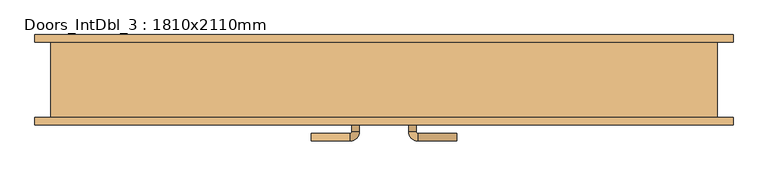
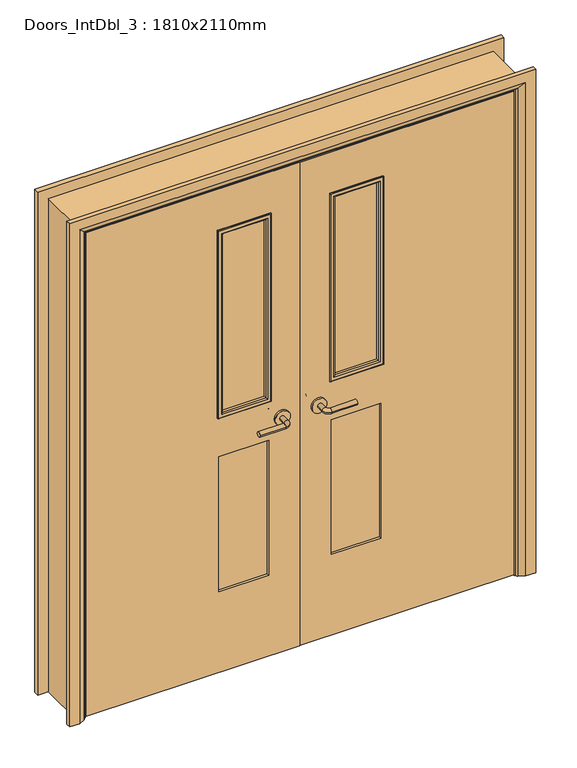
"""IFC4 building model written with IfcOpenShell, lengths in millimetres: door geometry, Doors_IntDbl_3 : 1810x2110mm."""

from ifc_helpers import new_model, si_unit, point, frame, frame_2d, origin, place, context, project, spatial, polyline, circle_curve, ellipse_curve, trimmed, segment, composite_curve, outline, extrude, faceted_brep, source, transform, mapped, element, save
from ifc_brep_helpers import plane_surface, cylinder_surface, revolved_surface, advanced_brep


def doors_intdbl_3_1810x2110mm_301b02ef(model_context):
    return source(origin(), model_context, "Body", "SolidModel", [
        advanced_brep(
        [(-66.5, -61.6, 1007.0), (-86.5, -61.6, 1007.0), (-86.5, -31.6, 1007.0), (-66.5, -31.6, 1007.0), (-91.5, -26.6, 1007.0), (-91.5, -6.6, 1007.0), (-196.5, -6.6, 1007.0), (-196.5, -26.6, 1007.0)],
        [
            (0, 1, circle_curve(frame((-76.5, -61.6, 1007.0), z_axis=(0.0, -1.0, 0.0), x_axis=(-1.0, 0.0, 0.0)), 10.0)),
            (1, 0, circle_curve(frame((-76.5, -61.6, 1007.0), z_axis=(0.0, -1.0, 0.0), x_axis=(-1.0, 0.0, 0.0)), 10.0)),
            (1, 2),
            (2, 3, circle_curve(frame((-76.5, -31.6, 1007.0), z_axis=(0.0, -1.0, 0.0), x_axis=(-1.0, 0.0, 0.0)), 10.0)),
            (3, 0),
            (3, 2, circle_curve(frame((-76.5, -31.6, 1007.0), z_axis=(0.0, -1.0, 0.0), x_axis=(-1.0, 0.0, 0.0)), 10.0)),
            (4, 5, circle_curve(frame((-91.5, -16.6, 1007.0), z_axis=(1.0, 0.0, 0.0), x_axis=(0.0, -1.0, 0.0)), 10.0)),
            (5, 3, circle_curve(frame((-91.5, -31.6, 1007.0), z_axis=(0.0, 0.0, -1.0), x_axis=(1.0, 0.0, 0.0)), 25.0)),
            (2, 4, circle_curve(frame((-91.5, -31.6, 1007.0), z_axis=(0.0, 0.0, 1.0), x_axis=(1.0, 0.0, 0.0)), 5.0)),
            (5, 4, circle_curve(frame((-91.5, -16.6, 1007.0), z_axis=(1.0, 0.0, 0.0), x_axis=(0.0, -1.0, 0.0)), 10.0)),
            (6, 7, circle_curve(frame((-196.5, -16.6, 1007.0), z_axis=(-1.0, 0.0, 0.0), x_axis=(0.0, -1.0, 0.0)), 10.0)),
            (7, 6, circle_curve(frame((-196.5, -16.6, 1007.0), z_axis=(-1.0, 0.0, 0.0), x_axis=(0.0, -1.0, 0.0)), 10.0)),
            (4, 7),
            (6, 5),
        ],
        [
            plane_surface(frame((-76.5, -61.6, 1007.0), z_axis=(0.0, -1.0, 0.0), x_axis=(0.0, 0.0, 1.0))),
            cylinder_surface(frame((-76.5, -61.6, 1007.0), z_axis=(0.0, -1.0, 0.0), x_axis=(-1.0, 0.0, 0.0)), 10.0),
            revolved_surface(trimmed(ellipse_curve(frame((-76.5, -31.6, 1007.0), z_axis=(0.0, 1.0, 0.0), x_axis=(-1.0, 0.0, 0.0)), 10.0, 10.0), [point((-66.5, -31.6, 1007.0))], [point((-86.5, -31.6, 1007.0))], True, "CARTESIAN"), (-91.5, -31.6, 1007.0), (0.0, 0.0, -1.0)),
            revolved_surface(trimmed(ellipse_curve(frame((-76.5, -31.6, 1007.0), z_axis=(0.0, 1.0, 0.0), x_axis=(-1.0, 0.0, 0.0)), 10.0, 10.0), [point((-86.5, -31.6, 1007.0))], [point((-66.5, -31.6, 1007.0))], True, "CARTESIAN"), (-91.5, -31.6, 1007.0), (0.0, 0.0, -1.0)),
            plane_surface(frame((-196.5, -16.6, 1007.0), z_axis=(-1.0, 0.0, 0.0), x_axis=(0.0, 0.0, 1.0))),
            cylinder_surface(frame((-91.5, -16.6, 1007.0), z_axis=(1.0, 0.0, 0.0), x_axis=(0.0, -1.0, 0.0)), 10.0),
        ],
        [
            (0, [[1, 2]]),
            (1, [[3, 4, 5, -2]]),
            (1, [[-5, 6, -3, -1]]),
            (2, [[7, 8, -4, 9]]),
            (3, [[10, -9, -6, -8]]),
            (4, [[11, 12]]),
            (5, [[13, -11, 14, -7]]),
            (5, [[-14, -12, -13, -10]]),
        ],
    ),
        extrude(outline(composite_curve([segment(trimmed(circle_curve(frame_2d((1007.0, -74.0)), 30.0), [point((1007.0, -44.0))], [point((1007.0, -104.0))], False, "CARTESIAN"), True, "CONTINUOUS"), segment(trimmed(circle_curve(frame_2d((1007.0, -74.0)), 30.0), [point((1007.0, -104.0))], [point((1007.0, -44.0))], False, "CARTESIAN"), True, "CONTINUOUS")], self_intersect=False)), frame((0.0, -69.6, 0.0), z_axis=(0.0, 1.0, 0.0), x_axis=(0.0, 0.0, 1.0)), (0.0, 0.0, 1.0), 8.0),
        advanced_brep(
        [(-66.5, -109.6, 1007.0), (-86.5, -109.6, 1007.0), (-66.5, -139.6, 1007.0), (-86.5, -139.6, 1007.0), (-91.5, -144.6, 1007.0), (-91.5, -164.6, 1007.0), (-196.5, -164.6, 1007.0), (-196.5, -144.6, 1007.0)],
        [
            (0, 1, circle_curve(frame((-76.5, -109.6, 1007.0), z_axis=(0.0, 1.0, 0.0), x_axis=(-1.0, 0.0, 0.0)), 10.0)),
            (1, 0, circle_curve(frame((-76.5, -109.6, 1007.0), z_axis=(0.0, 1.0, 0.0), x_axis=(-1.0, 0.0, 0.0)), 10.0)),
            (0, 2),
            (2, 3, circle_curve(frame((-76.5, -139.6, 1007.0), z_axis=(0.0, 1.0, 0.0), x_axis=(-1.0, 0.0, 0.0)), 10.0)),
            (3, 1),
            (3, 2, circle_curve(frame((-76.5, -139.6, 1007.0), z_axis=(0.0, 1.0, 0.0), x_axis=(-1.0, 0.0, 0.0)), 10.0)),
            (4, 3, circle_curve(frame((-91.5, -139.6, 1007.0), z_axis=(0.0, 0.0, 1.0), x_axis=(1.0, 0.0, 0.0)), 5.0)),
            (2, 5, circle_curve(frame((-91.5, -139.6, 1007.0), z_axis=(0.0, 0.0, -1.0), x_axis=(1.0, 0.0, 0.0)), 25.0)),
            (5, 4, circle_curve(frame((-91.5, -154.6, 1007.0), z_axis=(1.0, 0.0, 0.0), x_axis=(0.0, 1.0, 0.0)), 10.0)),
            (4, 5, circle_curve(frame((-91.5, -154.6, 1007.0), z_axis=(1.0, 0.0, 0.0), x_axis=(0.0, 1.0, 0.0)), 10.0)),
            (6, 7, circle_curve(frame((-196.5, -154.6, 1007.0), z_axis=(-1.0, 0.0, 0.0), x_axis=(0.0, 1.0, 0.0)), 10.0)),
            (7, 6, circle_curve(frame((-196.5, -154.6, 1007.0), z_axis=(-1.0, 0.0, 0.0), x_axis=(0.0, 1.0, 0.0)), 10.0)),
            (5, 6),
            (7, 4),
        ],
        [
            plane_surface(frame((-76.5, -109.6, 1007.0), z_axis=(0.0, 1.0, 0.0), x_axis=(0.0, 0.0, 1.0))),
            cylinder_surface(frame((-76.5, -109.6, 1007.0), z_axis=(0.0, 1.0, 0.0), x_axis=(-1.0, 0.0, 0.0)), 10.0),
            revolved_surface(trimmed(ellipse_curve(frame((-76.5, -139.6, 1007.0), z_axis=(0.0, 1.0, 0.0), x_axis=(-1.0, 0.0, 0.0)), 10.0, 10.0), [point((-66.5, -139.6, 1007.0))], [point((-86.5, -139.6, 1007.0))], True, "CARTESIAN"), (-91.5, -139.6, 1007.0), (0.0, 0.0, -1.0)),
            revolved_surface(trimmed(ellipse_curve(frame((-76.5, -139.6, 1007.0), z_axis=(0.0, 1.0, 0.0), x_axis=(-1.0, 0.0, 0.0)), 10.0, 10.0), [point((-86.5, -139.6, 1007.0))], [point((-66.5, -139.6, 1007.0))], True, "CARTESIAN"), (-91.5, -139.6, 1007.0), (0.0, 0.0, -1.0)),
            plane_surface(frame((-196.5, -154.6, 1007.0), z_axis=(-1.0, 0.0, 0.0), x_axis=(0.0, 0.0, 1.0))),
            cylinder_surface(frame((-91.5, -154.6, 1007.0), z_axis=(1.0, 0.0, 0.0), x_axis=(0.0, 1.0, 0.0)), 10.0),
        ],
        [
            (0, [[1, 2]]),
            (1, [[-1, 3, 4, 5]]),
            (1, [[-2, -5, 6, -3]]),
            (2, [[7, -4, 8, 9]]),
            (3, [[-8, -6, -7, 10]]),
            (4, [[11, 12]]),
            (5, [[-9, 13, -12, 14]]),
            (5, [[-10, -14, -11, -13]]),
        ],
    ),
        extrude(outline(composite_curve([segment(trimmed(circle_curve(frame_2d((1007.0, -74.0)), 30.0), [point((1007.0, -44.0))], [point((1007.0, -104.0))], False, "CARTESIAN"), True, "CONTINUOUS"), segment(trimmed(circle_curve(frame_2d((1007.0, -74.0)), 30.0), [point((1007.0, -104.0))], [point((1007.0, -44.0))], False, "CARTESIAN"), True, "CONTINUOUS")], self_intersect=False)), frame((0.0, -109.6, 0.0), z_axis=(0.0, 1.0, 0.0), x_axis=(0.0, 0.0, 1.0)), (0.0, 0.0, 1.0), 8.0),
        advanced_brep(
        [(66.5, -61.6, 1007.0), (86.5, -61.6, 1007.0), (66.5, -31.6, 1007.0), (86.5, -31.6, 1007.0), (91.5, -26.6, 1007.0), (91.5, -6.6, 1007.0), (196.5, -6.6, 1007.0), (196.5, -26.6, 1007.0)],
        [
            (0, 1, circle_curve(frame((76.5, -61.6, 1007.0), z_axis=(0.0, -1.0, 0.0), x_axis=(1.0, 0.0, 0.0)), 10.0)),
            (1, 0, circle_curve(frame((76.5, -61.6, 1007.0), z_axis=(0.0, -1.0, 0.0), x_axis=(1.0, 0.0, 0.0)), 10.0)),
            (0, 2),
            (2, 3, circle_curve(frame((76.5, -31.6, 1007.0), z_axis=(0.0, -1.0, 0.0), x_axis=(1.0, 0.0, 0.0)), 10.0)),
            (3, 1),
            (3, 2, circle_curve(frame((76.5, -31.6, 1007.0), z_axis=(0.0, -1.0, 0.0), x_axis=(1.0, 0.0, 0.0)), 10.0)),
            (4, 3, circle_curve(frame((91.5, -31.6, 1007.0), z_axis=(0.0, 0.0, 1.0), x_axis=(-1.0, 0.0, 0.0)), 5.0)),
            (2, 5, circle_curve(frame((91.5, -31.6, 1007.0), z_axis=(0.0, 0.0, -1.0), x_axis=(-1.0, 0.0, 0.0)), 25.0)),
            (5, 4, circle_curve(frame((91.5, -16.6, 1007.0), z_axis=(-1.0, 0.0, 0.0), x_axis=(0.0, -1.0, 0.0)), 10.0)),
            (4, 5, circle_curve(frame((91.5, -16.6, 1007.0), z_axis=(-1.0, 0.0, 0.0), x_axis=(0.0, -1.0, 0.0)), 10.0)),
            (6, 7, circle_curve(frame((196.5, -16.6, 1007.0), z_axis=(1.0, 0.0, 0.0), x_axis=(0.0, -1.0, 0.0)), 10.0)),
            (7, 6, circle_curve(frame((196.5, -16.6, 1007.0), z_axis=(1.0, 0.0, 0.0), x_axis=(0.0, -1.0, 0.0)), 10.0)),
            (5, 6),
            (7, 4),
        ],
        [
            plane_surface(frame((76.5, -61.6, 1007.0), z_axis=(0.0, -1.0, 0.0), x_axis=(0.0, 0.0, 1.0))),
            cylinder_surface(frame((76.5, -61.6, 1007.0), z_axis=(0.0, -1.0, 0.0), x_axis=(1.0, 0.0, 0.0)), 10.0),
            revolved_surface(trimmed(ellipse_curve(frame((76.5, -31.6, 1007.0), z_axis=(0.0, -1.0, 0.0), x_axis=(1.0, 0.0, 0.0)), 10.0, 10.0), [point((66.5, -31.6, 1007.0))], [point((86.5, -31.6, 1007.0))], True, "CARTESIAN"), (91.5, -31.6, 1007.0), (0.0, 0.0, -1.0)),
            revolved_surface(trimmed(ellipse_curve(frame((76.5, -31.6, 1007.0), z_axis=(0.0, -1.0, 0.0), x_axis=(1.0, 0.0, 0.0)), 10.0, 10.0), [point((86.5, -31.6, 1007.0))], [point((66.5, -31.6, 1007.0))], True, "CARTESIAN"), (91.5, -31.6, 1007.0), (0.0, 0.0, -1.0)),
            plane_surface(frame((196.5, -16.6, 1007.0), z_axis=(1.0, 0.0, 0.0), x_axis=(0.0, 0.0, 1.0))),
            cylinder_surface(frame((91.5, -16.6, 1007.0), z_axis=(-1.0, 0.0, 0.0), x_axis=(0.0, -1.0, 0.0)), 10.0),
        ],
        [
            (0, [[1, 2]]),
            (1, [[-1, 3, 4, 5]]),
            (1, [[-2, -5, 6, -3]]),
            (2, [[7, -4, 8, 9]]),
            (3, [[-8, -6, -7, 10]]),
            (4, [[11, 12]]),
            (5, [[-9, 13, -12, 14]]),
            (5, [[-10, -14, -11, -13]]),
        ],
    ),
        extrude(outline(composite_curve([segment(trimmed(circle_curve(frame_2d((1007.0, 74.0)), 30.0), [point((1007.0, 44.0))], [point((1007.0, 104.0))], False, "CARTESIAN"), True, "CONTINUOUS"), segment(trimmed(circle_curve(frame_2d((1007.0, 74.0)), 30.0), [point((1007.0, 104.0))], [point((1007.0, 44.0))], False, "CARTESIAN"), True, "CONTINUOUS")], self_intersect=False)), frame((0.0, -69.6, 0.0), z_axis=(0.0, 1.0, 0.0), x_axis=(0.0, 0.0, 1.0)), (0.0, 0.0, 1.0), 8.0),
        advanced_brep(
        [(66.5, -109.6, 1007.0), (86.5, -109.6, 1007.0), (86.5, -139.6, 1007.0), (66.5, -139.6, 1007.0), (91.5, -144.6, 1007.0), (91.5, -164.6, 1007.0), (196.5, -164.6, 1007.0), (196.5, -144.6, 1007.0)],
        [
            (0, 1, circle_curve(frame((76.5, -109.6, 1007.0), z_axis=(0.0, 1.0, 0.0), x_axis=(1.0, 0.0, 0.0)), 10.0)),
            (1, 0, circle_curve(frame((76.5, -109.6, 1007.0), z_axis=(0.0, 1.0, 0.0), x_axis=(1.0, 0.0, 0.0)), 10.0)),
            (1, 2),
            (2, 3, circle_curve(frame((76.5, -139.6, 1007.0), z_axis=(0.0, 1.0, 0.0), x_axis=(1.0, 0.0, 0.0)), 10.0)),
            (3, 0),
            (3, 2, circle_curve(frame((76.5, -139.6, 1007.0), z_axis=(0.0, 1.0, 0.0), x_axis=(1.0, 0.0, 0.0)), 10.0)),
            (4, 5, circle_curve(frame((91.5, -154.6, 1007.0), z_axis=(-1.0, 0.0, 0.0), x_axis=(0.0, 1.0, 0.0)), 10.0)),
            (5, 3, circle_curve(frame((91.5, -139.6, 1007.0), z_axis=(0.0, 0.0, -1.0), x_axis=(-1.0, 0.0, 0.0)), 25.0)),
            (2, 4, circle_curve(frame((91.5, -139.6, 1007.0), z_axis=(0.0, 0.0, 1.0), x_axis=(-1.0, 0.0, 0.0)), 5.0)),
            (5, 4, circle_curve(frame((91.5, -154.6, 1007.0), z_axis=(-1.0, 0.0, 0.0), x_axis=(0.0, 1.0, 0.0)), 10.0)),
            (6, 7, circle_curve(frame((196.5, -154.6, 1007.0), z_axis=(1.0, 0.0, 0.0), x_axis=(0.0, 1.0, 0.0)), 10.0)),
            (7, 6, circle_curve(frame((196.5, -154.6, 1007.0), z_axis=(1.0, 0.0, 0.0), x_axis=(0.0, 1.0, 0.0)), 10.0)),
            (4, 7),
            (6, 5),
        ],
        [
            plane_surface(frame((76.5, -109.6, 1007.0), z_axis=(0.0, 1.0, 0.0), x_axis=(0.0, 0.0, 1.0))),
            cylinder_surface(frame((76.5, -109.6, 1007.0), z_axis=(0.0, 1.0, 0.0), x_axis=(1.0, 0.0, 0.0)), 10.0),
            revolved_surface(trimmed(ellipse_curve(frame((76.5, -139.6, 1007.0), z_axis=(0.0, -1.0, 0.0), x_axis=(1.0, 0.0, 0.0)), 10.0, 10.0), [point((66.5, -139.6, 1007.0))], [point((86.5, -139.6, 1007.0))], True, "CARTESIAN"), (91.5, -139.6, 1007.0), (0.0, 0.0, -1.0)),
            revolved_surface(trimmed(ellipse_curve(frame((76.5, -139.6, 1007.0), z_axis=(0.0, -1.0, 0.0), x_axis=(1.0, 0.0, 0.0)), 10.0, 10.0), [point((86.5, -139.6, 1007.0))], [point((66.5, -139.6, 1007.0))], True, "CARTESIAN"), (91.5, -139.6, 1007.0), (0.0, 0.0, -1.0)),
            plane_surface(frame((196.5, -154.6, 1007.0), z_axis=(1.0, 0.0, 0.0), x_axis=(0.0, 0.0, 1.0))),
            cylinder_surface(frame((91.5, -154.6, 1007.0), z_axis=(-1.0, 0.0, 0.0), x_axis=(0.0, 1.0, 0.0)), 10.0),
        ],
        [
            (0, [[1, 2]]),
            (1, [[3, 4, 5, -2]]),
            (1, [[-5, 6, -3, -1]]),
            (2, [[7, 8, -4, 9]]),
            (3, [[10, -9, -6, -8]]),
            (4, [[11, 12]]),
            (5, [[13, -11, 14, -7]]),
            (5, [[-14, -12, -13, -10]]),
        ],
    ),
        extrude(outline(composite_curve([segment(trimmed(circle_curve(frame_2d((1007.0, 74.0)), 30.0), [point((1007.0, 44.0))], [point((1007.0, 104.0))], False, "CARTESIAN"), True, "CONTINUOUS"), segment(trimmed(circle_curve(frame_2d((1007.0, 74.0)), 30.0), [point((1007.0, 104.0))], [point((1007.0, 44.0))], False, "CARTESIAN"), True, "CONTINUOUS")], self_intersect=False)), frame((0.0, -109.6, 0.0), z_axis=(0.0, 1.0, 0.0), x_axis=(0.0, 0.0, 1.0)), (0.0, 0.0, 1.0), 8.0),
        extrude(outline(polyline([(2102.0, -897.0), (0.0, -897.0), (0.0, -865.0), (2070.0, -865.0), (2070.0, 865.0), (0.0, 865.0), (0.0, 897.0), (2102.0, 897.0), (2102.0, -897.0)])), frame((0.0, -101.6, 0.0), z_axis=(0.0, 1.0, 0.0), x_axis=(0.0, 0.0, 1.0)), (0.0, 0.0, 1.0), 203.2),
        faceted_brep([(-846.0, -66.6, 0.0), (-865.0, -66.6, 0.0), (-865.0, -34.6, 0.0), (-846.0, -34.6, 0.0), (-846.0, -34.6, 2051.0), (-846.0, -66.6, 2051.0), (-865.0, -34.6, 2070.0), (-865.0, -66.6, 2070.0), (846.0, -66.6, 0.0), (846.0, -34.6, 0.0), (865.0, -34.6, 0.0), (865.0, -66.6, 0.0), (846.0, -66.6, 2051.0), (865.0, -66.6, 2070.0), (865.0, -34.6, 2070.0), (846.0, -34.6, 2051.0)], [[[0, 1, 2, 3]], [[3, 4, 5, 0]], [[2, 6, 4, 3]], [[1, 7, 6, 2]], [[0, 5, 7, 1]], [[8, 9, 10, 11]], [[12, 8, 11, 13]], [[13, 11, 10, 14]], [[14, 10, 9, 15]], [[15, 9, 8, 12]], [[4, 15, 12, 5]], [[6, 14, 15, 4]], [[7, 13, 14, 6]], [[5, 12, 13, 7]]]),
        advanced_brep(
        [(940.0, -121.6, 0.0), (900.0, -121.6, 0.0), (874.0, -107.6, 0.0), (870.0, -101.6, 0.0), (940.0, -101.6, 0.0), (940.0, -101.6, 2145.0), (940.0, -121.6, 2145.0), (870.0, -101.6, 2075.0), (-870.0, -101.6, 2075.0), (-870.0, -101.6, 0.0), (-940.0, -101.6, 0.0), (-940.0, -101.6, 2145.0), (874.0, -107.6, 2079.0), (900.0, -121.6, 2105.0), (-940.0, -121.6, 2145.0), (-940.0, -121.6, 0.0), (-900.0, -121.6, 0.0), (-900.0, -121.6, 2105.0), (-874.0, -107.6, 0.0), (-874.0, -107.6, 2079.0)],
        [
            (0, 1),
            (1, 2),
            (2, 3, circle_curve(frame((878.0, -100.6, 0.0), z_axis=(0.0, 0.0, -1.0), x_axis=(1.0, 0.0, 0.0)), 8.0622577)),
            (3, 4),
            (4, 0),
            (4, 5),
            (5, 6),
            (6, 0),
            (3, 7),
            (7, 8),
            (8, 9),
            (9, 10),
            (10, 11),
            (11, 5),
            (2, 12),
            (12, 7, ellipse_curve(frame((878.0, -100.6, 2083.0), z_axis=(0.7071067811865475, 0.0, -0.7071067811865475), x_axis=(-0.7071067811865474, 0.0, -0.7071067811865476)), 11.4017543, 8.0622577)),
            (1, 13),
            (13, 12),
            (6, 14),
            (14, 15),
            (15, 16),
            (16, 17),
            (17, 13),
            (10, 15),
            (14, 11),
            (9, 18, circle_curve(frame((-878.0, -100.6, 0.0), z_axis=(0.0, 0.0, -1.0), x_axis=(-1.0, 0.0, 0.0)), 8.0622577)),
            (18, 16),
            (19, 18),
            (8, 19, ellipse_curve(frame((-878.0, -100.6, 2083.0), z_axis=(-0.7071067811865475, 0.0, -0.7071067811865475), x_axis=(-0.7071067811865474, 0.0, 0.7071067811865476)), 11.4017543, 8.0622577)),
            (19, 17),
            (12, 19),
        ],
        [
            plane_surface(frame((870.0, -101.6, 0.0), z_axis=(0.0, 0.0, -1.0), x_axis=(0.0, 1.0, 0.0))),
            plane_surface(frame((940.0, -121.6, 0.0), z_axis=(1.0, 0.0, 0.0), x_axis=(0.0, 0.0, 1.0))),
            plane_surface(frame((940.0, -101.6, 0.0), z_axis=(0.0, 1.0, 0.0), x_axis=(0.0, 0.0, 1.0))),
            cylinder_surface(frame((878.0, -100.6, 0.0), z_axis=(0.0, 0.0, -1.0), x_axis=(1.0, 0.0, 0.0)), 8.0622577),
            plane_surface(frame((874.0, -107.6, 0.0), z_axis=(-0.4740998230350126, -0.8804710999221779, 0.0), x_axis=(0.0, 0.0, 1.0))),
            plane_surface(frame((900.0, -121.6, 0.0), z_axis=(0.0, -1.0, 0.0), x_axis=(0.0, 0.0, 1.0))),
            plane_surface(frame((-940.0, -121.6, 2145.0), z_axis=(-1.0, 0.0, 0.0), x_axis=(0.0, 0.0, -1.0))),
            plane_surface(frame((-870.0, -101.6, 0.0), z_axis=(0.0, 0.0, -1.0), x_axis=(0.0, 1.0, 0.0))),
            cylinder_surface(frame((-878.0, -100.6, 2075.0), z_axis=(0.0, 0.0, 1.0), x_axis=(-1.0, 0.0, 0.0)), 8.0622577),
            plane_surface(frame((-874.0, -107.6, 2079.0), z_axis=(0.4740998230350183, -0.8804710999221749, 0.0), x_axis=(0.0, 0.0, -1.0))),
            plane_surface(frame((940.0, -121.6, 2145.0), z_axis=(0.0, 0.0, 1.0), x_axis=(-1.0, 0.0, 0.0))),
            cylinder_surface(frame((870.0, -100.6, 2083.0), z_axis=(1.0, 0.0, 0.0), x_axis=(0.0, 0.0, 1.0)), 8.0622577),
            plane_surface(frame((874.0, -107.6, 2079.0), z_axis=(0.0, -0.8804710999221763, -0.4740998230350154), x_axis=(-1.0, 0.0, 0.0))),
        ],
        [
            (0, [[1, 2, 3, 4, 5]]),
            (1, [[6, 7, 8, -5]]),
            (2, [[9, 10, 11, 12, 13, 14, -6, -4]]),
            (3, [[15, 16, -9, -3]]),
            (4, [[17, 18, -15, -2]]),
            (5, [[-8, 19, 20, 21, 22, 23, -17, -1]]),
            (6, [[-13, 24, -20, 25]]),
            (7, [[-24, -12, 26, 27, -21]]),
            (8, [[28, -26, -11, 29]]),
            (9, [[-22, -27, -28, 30]]),
            (10, [[-14, -25, -19, -7]]),
            (11, [[31, -29, -10, -16]]),
            (12, [[-23, -30, -31, -18]]),
        ],
    ),
        advanced_brep(
        [(-940.0, 121.6, 0.0), (-900.0, 121.6, 0.0), (-874.0, 107.6, 0.0), (-870.0, 101.6, 0.0), (-940.0, 101.6, 0.0), (-940.0, 101.6, 2145.0), (-940.0, 121.6, 2145.0), (-870.0, 101.6, 2075.0), (870.0, 101.6, 2075.0), (870.0, 101.6, 0.0), (940.0, 101.6, 0.0), (940.0, 101.6, 2145.0), (-874.0, 107.6, 2079.0), (-900.0, 121.6, 2105.0), (940.0, 121.6, 2145.0), (940.0, 121.6, 0.0), (900.0, 121.6, 0.0), (900.0, 121.6, 2105.0), (874.0, 107.6, 0.0), (874.0, 107.6, 2079.0)],
        [
            (0, 1),
            (1, 2),
            (2, 3, circle_curve(frame((-878.0, 100.6, 0.0), z_axis=(0.0, 0.0, -1.0), x_axis=(-1.0, 0.0, 0.0)), 8.0622577)),
            (3, 4),
            (4, 0),
            (4, 5),
            (5, 6),
            (6, 0),
            (3, 7),
            (7, 8),
            (8, 9),
            (9, 10),
            (10, 11),
            (11, 5),
            (2, 12),
            (12, 7, ellipse_curve(frame((-878.0, 100.6, 2083.0), z_axis=(-0.7071067811865475, 0.0, -0.7071067811865475), x_axis=(0.7071067811865474, 0.0, -0.7071067811865476)), 11.4017543, 8.0622577)),
            (1, 13),
            (13, 12),
            (6, 14),
            (14, 15),
            (15, 16),
            (16, 17),
            (17, 13),
            (10, 15),
            (14, 11),
            (9, 18, circle_curve(frame((878.0, 100.6, 0.0), z_axis=(0.0, 0.0, -1.0), x_axis=(1.0, 0.0, 0.0)), 8.0622577)),
            (18, 16),
            (19, 18),
            (8, 19, ellipse_curve(frame((878.0, 100.6, 2083.0), z_axis=(0.7071067811865475, 0.0, -0.7071067811865475), x_axis=(0.7071067811865474, 0.0, 0.7071067811865476)), 11.4017543, 8.0622577)),
            (19, 17),
            (12, 19),
        ],
        [
            plane_surface(frame((-870.0, 101.6, 0.0), z_axis=(0.0, 0.0, -1.0), x_axis=(0.0, 1.0, 0.0))),
            plane_surface(frame((-940.0, 121.6, 0.0), z_axis=(-1.0, 0.0, 0.0), x_axis=(0.0, 0.0, 1.0))),
            plane_surface(frame((-940.0, 101.6, 0.0), z_axis=(0.0, -1.0, 0.0), x_axis=(0.0, 0.0, 1.0))),
            cylinder_surface(frame((-878.0, 100.6, 0.0), z_axis=(0.0, 0.0, -1.0), x_axis=(-1.0, 0.0, 0.0)), 8.0622577),
            plane_surface(frame((-874.0, 107.6, 0.0), z_axis=(0.4740998230350183, 0.8804710999221749, 0.0), x_axis=(0.0, 0.0, 1.0))),
            plane_surface(frame((-900.0, 121.6, 0.0), z_axis=(0.0, 1.0, 0.0), x_axis=(0.0, 0.0, 1.0))),
            plane_surface(frame((940.0, 121.6, 2145.0), z_axis=(1.0, 0.0, 0.0), x_axis=(0.0, 0.0, -1.0))),
            plane_surface(frame((870.0, 101.6, 0.0), z_axis=(0.0, 0.0, -1.0), x_axis=(0.0, 1.0, 0.0))),
            cylinder_surface(frame((878.0, 100.6, 2075.0), z_axis=(0.0, 0.0, 1.0), x_axis=(1.0, 0.0, 0.0)), 8.0622577),
            plane_surface(frame((874.0, 107.6, 2079.0), z_axis=(-0.4740998230350183, 0.8804710999221749, 0.0), x_axis=(0.0, 0.0, -1.0))),
            plane_surface(frame((-940.0, 121.6, 2145.0), z_axis=(0.0, 0.0, 1.0), x_axis=(1.0, 0.0, 0.0))),
            cylinder_surface(frame((-870.0, 100.6, 2083.0), z_axis=(-1.0, 0.0, 0.0), x_axis=(0.0, 0.0, 1.0)), 8.0622577),
            plane_surface(frame((-874.0, 107.6, 2079.0), z_axis=(0.0, 0.8804710999221749, -0.4740998230350183), x_axis=(1.0, 0.0, 0.0))),
        ],
        [
            (0, [[1, 2, 3, 4, 5]]),
            (1, [[6, 7, 8, -5]]),
            (2, [[9, 10, 11, 12, 13, 14, -6, -4]]),
            (3, [[15, 16, -9, -3]]),
            (4, [[17, 18, -15, -2]]),
            (5, [[-8, 19, 20, 21, 22, 23, -17, -1]]),
            (6, [[-13, 24, -20, 25]]),
            (7, [[-24, -12, 26, 27, -21]]),
            (8, [[28, -26, -11, 29]]),
            (9, [[-22, -27, -28, 30]]),
            (10, [[-14, -25, -19, -7]]),
            (11, [[31, -29, -10, -16]]),
            (12, [[-23, -30, -31, -18]]),
        ],
    ),
        extrude(outline(polyline([(5.753223, 862.0), (2067.0, 862.0), (2067.0, 1.5), (5.753223, 1.5), (5.753223, 862.0)]), holes=[polyline([(1885.0, 126.5), (1885.0, 326.5), (1100.0, 326.5), (1100.0, 126.5), (1885.0, 126.5)]), polyline([(925.0, 326.5), (350.0, 326.5), (350.0, 126.5), (925.0, 126.5), (925.0, 326.5)])]), frame((0.0, -101.6, 0.0), z_axis=(0.0, 1.0, 0.0), x_axis=(0.0, 0.0, 1.0)), (0.0, 0.0, 1.0), 32.0),
        extrude(outline(polyline([(5.753223, -862.0), (5.753223, -1.5), (2067.0, -1.5), (2067.0, -862.0), (5.753223, -862.0)]), holes=[polyline([(1885.0, -326.5), (1885.0, -126.5), (1100.0, -126.5), (1100.0, -326.5), (1885.0, -326.5)]), polyline([(925.0, -126.5), (350.0, -126.5), (350.0, -326.5), (925.0, -326.5), (925.0, -126.5)])]), frame((0.0, -101.6, 0.0), z_axis=(0.0, 1.0, 0.0), x_axis=(0.0, 0.0, 1.0)), (0.0, 0.0, 1.0), 32.0),
        extrude(outline(polyline([(326.5, -79.6), (326.5, -91.6), (126.5, -91.6), (126.5, -79.6), (326.5, -79.6)])), frame((0.0, 0.0, 1100.0), z_axis=(0.0, 0.0, 1.0), x_axis=(1.0, 0.0, 0.0)), (0.0, 0.0, 1.0), 785.0),
        extrude(outline(polyline([(326.5, -79.6), (326.5, -91.6), (126.5, -91.6), (126.5, -79.6), (326.5, -79.6)])), frame((0.0, 0.0, 350.0), z_axis=(0.0, 0.0, 1.0), x_axis=(1.0, 0.0, 0.0)), (0.0, 0.0, 1.0), 575.0),
        extrude(outline(polyline([(-126.5, -79.6), (-126.5, -91.6), (-326.5, -91.6), (-326.5, -79.6), (-126.5, -79.6)])), frame((0.0, 0.0, 350.0), z_axis=(0.0, 0.0, 1.0), x_axis=(1.0, 0.0, 0.0)), (0.0, 0.0, 1.0), 575.0),
        extrude(outline(polyline([(-126.5, -79.6), (-126.5, -91.6), (-326.5, -91.6), (-326.5, -79.6), (-126.5, -79.6)])), frame((0.0, 0.0, 1100.0), z_axis=(0.0, 0.0, 1.0), x_axis=(1.0, 0.0, 0.0)), (0.0, 0.0, 1.0), 785.0),
        advanced_brep(
        [(-326.5, -91.6, 1885.0), (-326.5, -91.6, 1100.0), (-326.5, -101.6, 1100.0), (-326.5, -101.6, 1885.0), (-314.5, -102.6, 1873.0), (-314.5, -102.6, 1112.0), (-314.5, -91.6, 1112.0), (-314.5, -91.6, 1873.0), (-319.5, -107.6, 1878.0), (-319.5, -107.6, 1107.0), (-334.5, -105.6, 1893.0), (-334.5, -105.6, 1092.0), (-332.5, -107.6, 1094.0), (-332.5, -107.6, 1891.0), (-334.5, -101.6, 1893.0), (-334.5, -101.6, 1092.0), (-126.5, -91.6, 1100.0), (-126.5, -101.6, 1100.0), (-138.5, -102.6, 1112.0), (-138.5, -91.6, 1112.0), (-133.5, -107.6, 1107.0), (-118.5, -105.6, 1092.0), (-120.5, -107.6, 1094.0), (-118.5, -101.6, 1092.0), (-126.5, -91.6, 1885.0), (-126.5, -101.6, 1885.0), (-138.5, -102.6, 1873.0), (-138.5, -91.6, 1873.0), (-133.5, -107.6, 1878.0), (-118.5, -105.6, 1893.0), (-120.5, -107.6, 1891.0), (-118.5, -101.6, 1893.0)],
        [
            (0, 1),
            (1, 2),
            (2, 3),
            (3, 0),
            (4, 5),
            (5, 6),
            (6, 7),
            (7, 4),
            (8, 9),
            (9, 5, ellipse_curve(frame((-319.5, -102.6, 1107.0), z_axis=(-0.7071067811865475, 0.0, 0.7071067811865475), x_axis=(0.7071067811865474, 0.0, 0.7071067811865476)), 7.0710678, 5.0)),
            (4, 8, ellipse_curve(frame((-319.5, -102.6, 1878.0), z_axis=(-0.7071067811865475, 0.0, -0.7071067811865475), x_axis=(-0.7071067811865474, 0.0, 0.7071067811865476)), 7.0710678, 5.0)),
            (10, 11),
            (11, 12, ellipse_curve(frame((-332.5, -105.6, 1094.0), z_axis=(-0.7071067811865475, 0.0, 0.7071067811865475), x_axis=(0.7071067811865474, 0.0, 0.7071067811865476)), 2.8284271, 2.0)),
            (12, 13),
            (13, 10, ellipse_curve(frame((-332.5, -105.6, 1891.0), z_axis=(-0.7071067811865475, 0.0, -0.7071067811865475), x_axis=(-0.7071067811865474, 0.0, 0.7071067811865476)), 2.8284271, 2.0)),
            (14, 15),
            (15, 11),
            (10, 14),
            (1, 16),
            (16, 17),
            (17, 2),
            (5, 18),
            (18, 19),
            (19, 6),
            (9, 20),
            (20, 18, ellipse_curve(frame((-133.5, -102.6, 1107.0), z_axis=(-0.7071067811865475, 0.0, -0.7071067811865475), x_axis=(-0.7071067811865476, 0.0, 0.7071067811865474)), 7.0710678, 5.0)),
            (11, 21),
            (21, 22, ellipse_curve(frame((-120.5, -105.6, 1094.0), z_axis=(-0.7071067811865475, 0.0, -0.7071067811865475), x_axis=(-0.7071067811865476, 0.0, 0.7071067811865474)), 2.8284271, 2.0)),
            (22, 12),
            (15, 23),
            (23, 21),
            (16, 24),
            (24, 25),
            (25, 17),
            (18, 26),
            (26, 27),
            (27, 19),
            (20, 28),
            (28, 26, ellipse_curve(frame((-133.5, -102.6, 1878.0), z_axis=(0.7071067811865475, 0.0, -0.7071067811865475), x_axis=(-0.7071067811865474, 0.0, -0.7071067811865476)), 7.0710678, 5.0)),
            (21, 29),
            (29, 30, ellipse_curve(frame((-120.5, -105.6, 1891.0), z_axis=(0.7071067811865475, 0.0, -0.7071067811865475), x_axis=(-0.7071067811865474, 0.0, -0.7071067811865476)), 2.8284271, 2.0)),
            (30, 22),
            (23, 31),
            (31, 29),
            (14, 31),
            (25, 3),
            (24, 0),
            (27, 7),
            (26, 4),
            (28, 8),
            (30, 13),
            (29, 10),
        ],
        [
            plane_surface(frame((-326.5, -101.6, 1885.0), z_axis=(-1.0, 0.0, 0.0), x_axis=(0.0, 0.0, -1.0))),
            plane_surface(frame((-314.5, -91.6, 1873.0), z_axis=(1.0, 0.0, 0.0), x_axis=(0.0, 0.0, -1.0))),
            cylinder_surface(frame((-319.5, -102.6, 1885.0), z_axis=(0.0, 0.0, 1.0), x_axis=(-1.0, 0.0, 0.0)), 5.0),
            cylinder_surface(frame((-332.5, -105.6, 1885.0), z_axis=(0.0, 0.0, 1.0), x_axis=(-1.0, 0.0, 0.0)), 2.0),
            plane_surface(frame((-334.5, -105.6, 1893.0), z_axis=(-1.0, 0.0, 0.0), x_axis=(0.0, 0.0, -1.0))),
            plane_surface(frame((-326.5, -101.6, 1100.0), z_axis=(0.0, 0.0, -1.0), x_axis=(1.0, 0.0, 0.0))),
            plane_surface(frame((-314.5, -91.6, 1112.0), z_axis=(0.0, 0.0, 1.0), x_axis=(1.0, 0.0, 0.0))),
            cylinder_surface(frame((-326.5, -102.6, 1107.0), z_axis=(-1.0, 0.0, 0.0), x_axis=(0.0, 0.0, -1.0)), 5.0),
            cylinder_surface(frame((-326.5, -105.6, 1094.0), z_axis=(-1.0, 0.0, 0.0), x_axis=(0.0, 0.0, -1.0)), 2.0),
            plane_surface(frame((-334.5, -105.6, 1092.0), z_axis=(0.0, 0.0, -1.0), x_axis=(1.0, 0.0, 0.0))),
            plane_surface(frame((-126.5, -101.6, 1100.0), z_axis=(1.0, 0.0, 0.0), x_axis=(0.0, 0.0, 1.0))),
            plane_surface(frame((-138.5, -91.6, 1112.0), z_axis=(-1.0, 0.0, 0.0), x_axis=(0.0, 0.0, 1.0))),
            cylinder_surface(frame((-133.5, -102.6, 1100.0), z_axis=(0.0, 0.0, -1.0), x_axis=(1.0, 0.0, 0.0)), 5.0),
            cylinder_surface(frame((-120.5, -105.6, 1100.0), z_axis=(0.0, 0.0, -1.0), x_axis=(1.0, 0.0, 0.0)), 2.0),
            plane_surface(frame((-118.5, -105.6, 1092.0), z_axis=(1.0, 0.0, 0.0), x_axis=(0.0, 0.0, 1.0))),
            plane_surface(frame((-118.5, -101.6, 1893.0), z_axis=(0.0, 1.0, 0.0), x_axis=(-1.0, 0.0, 0.0))),
            plane_surface(frame((-126.5, -101.6, 1885.0), z_axis=(0.0, 0.0, 1.0), x_axis=(-1.0, 0.0, 0.0))),
            plane_surface(frame((-126.5, -91.6, 1885.0), z_axis=(0.0, 1.0, 0.0), x_axis=(-1.0, 0.0, 0.0))),
            plane_surface(frame((-138.5, -91.6, 1873.0), z_axis=(0.0, 0.0, -1.0), x_axis=(-1.0, 0.0, 0.0))),
            cylinder_surface(frame((-126.5, -102.6, 1878.0), z_axis=(1.0, 0.0, 0.0), x_axis=(0.0, 0.0, 1.0)), 5.0),
            plane_surface(frame((-133.5, -107.6, 1878.0), z_axis=(0.0, -1.0, 0.0), x_axis=(-1.0, 0.0, 0.0))),
            cylinder_surface(frame((-126.5, -105.6, 1891.0), z_axis=(1.0, 0.0, 0.0), x_axis=(0.0, 0.0, 1.0)), 2.0),
            plane_surface(frame((-118.5, -105.6, 1893.0), z_axis=(0.0, 0.0, 1.0), x_axis=(-1.0, 0.0, 0.0))),
        ],
        [
            (0, [[1, 2, 3, 4]]),
            (1, [[5, 6, 7, 8]]),
            (2, [[9, 10, -5, 11]]),
            (3, [[12, 13, 14, 15]]),
            (4, [[16, 17, -12, 18]]),
            (5, [[19, 20, 21, -2]]),
            (6, [[22, 23, 24, -6]]),
            (7, [[25, 26, -22, -10]]),
            (8, [[27, 28, 29, -13]]),
            (9, [[30, 31, -27, -17]]),
            (10, [[32, 33, 34, -20]]),
            (11, [[35, 36, 37, -23]]),
            (12, [[38, 39, -35, -26]]),
            (13, [[40, 41, 42, -28]]),
            (14, [[43, 44, -40, -31]]),
            (15, [[-16, 45, -43, -30], [-3, -21, -34, 46]]),
            (16, [[47, -4, -46, -33]]),
            (17, [[-1, -47, -32, -19], [-7, -24, -37, 48]]),
            (18, [[49, -8, -48, -36]]),
            (19, [[50, -11, -49, -39]]),
            (20, [[-14, -29, -42, 51], [-9, -50, -38, -25]]),
            (21, [[52, -15, -51, -41]]),
            (22, [[-45, -18, -52, -44]]),
        ],
    ),
        advanced_brep(
        [(326.5, -91.6, 1100.0), (326.5, -91.6, 1885.0), (326.5, -101.6, 1885.0), (326.5, -101.6, 1100.0), (314.5, -102.6, 1112.0), (314.5, -102.6, 1873.0), (314.5, -91.6, 1873.0), (314.5, -91.6, 1112.0), (319.5, -107.6, 1107.0), (319.5, -107.6, 1878.0), (334.5, -105.6, 1092.0), (334.5, -105.6, 1893.0), (332.5, -107.6, 1891.0), (332.5, -107.6, 1094.0), (334.5, -101.6, 1092.0), (334.5, -101.6, 1893.0), (126.5, -91.6, 1885.0), (126.5, -101.6, 1885.0), (138.5, -102.6, 1873.0), (138.5, -91.6, 1873.0), (133.5, -107.6, 1878.0), (118.5, -105.6, 1893.0), (120.5, -107.6, 1891.0), (118.5, -101.6, 1893.0), (126.5, -91.6, 1100.0), (126.5, -101.6, 1100.0), (138.5, -102.6, 1112.0), (138.5, -91.6, 1112.0), (133.5, -107.6, 1107.0), (118.5, -105.6, 1092.0), (120.5, -107.6, 1094.0), (118.5, -101.6, 1092.0)],
        [
            (0, 1),
            (1, 2),
            (2, 3),
            (3, 0),
            (4, 5),
            (5, 6),
            (6, 7),
            (7, 4),
            (8, 9),
            (9, 5, ellipse_curve(frame((319.5, -102.6, 1878.0), z_axis=(0.7071067811865475, 0.0, -0.7071067811865475), x_axis=(-0.7071067811865474, 0.0, -0.7071067811865476)), 7.0710678, 5.0)),
            (4, 8, ellipse_curve(frame((319.5, -102.6, 1107.0), z_axis=(0.7071067811865475, 0.0, 0.7071067811865475), x_axis=(0.7071067811865474, 0.0, -0.7071067811865476)), 7.0710678, 5.0)),
            (10, 11),
            (11, 12, ellipse_curve(frame((332.5, -105.6, 1891.0), z_axis=(0.7071067811865475, 0.0, -0.7071067811865475), x_axis=(-0.7071067811865474, 0.0, -0.7071067811865476)), 2.8284271, 2.0)),
            (12, 13),
            (13, 10, ellipse_curve(frame((332.5, -105.6, 1094.0), z_axis=(0.7071067811865475, 0.0, 0.7071067811865475), x_axis=(0.7071067811865474, 0.0, -0.7071067811865476)), 2.8284271, 2.0)),
            (14, 15),
            (15, 11),
            (10, 14),
            (1, 16),
            (16, 17),
            (17, 2),
            (5, 18),
            (18, 19),
            (19, 6),
            (9, 20),
            (20, 18, ellipse_curve(frame((133.5, -102.6, 1878.0), z_axis=(0.7071067811865475, 0.0, 0.7071067811865475), x_axis=(0.7071067811865476, 0.0, -0.7071067811865474)), 7.0710678, 5.0)),
            (11, 21),
            (21, 22, ellipse_curve(frame((120.5, -105.6, 1891.0), z_axis=(0.7071067811865475, 0.0, 0.7071067811865475), x_axis=(0.7071067811865476, 0.0, -0.7071067811865474)), 2.8284271, 2.0)),
            (22, 12),
            (15, 23),
            (23, 21),
            (16, 24),
            (24, 25),
            (25, 17),
            (18, 26),
            (26, 27),
            (27, 19),
            (20, 28),
            (28, 26, ellipse_curve(frame((133.5, -102.6, 1107.0), z_axis=(-0.7071067811865475, 0.0, 0.7071067811865475), x_axis=(0.7071067811865474, 0.0, 0.7071067811865476)), 7.0710678, 5.0)),
            (21, 29),
            (29, 30, ellipse_curve(frame((120.5, -105.6, 1094.0), z_axis=(-0.7071067811865475, 0.0, 0.7071067811865475), x_axis=(0.7071067811865474, 0.0, 0.7071067811865476)), 2.8284271, 2.0)),
            (30, 22),
            (23, 31),
            (31, 29),
            (14, 31),
            (25, 3),
            (24, 0),
            (27, 7),
            (26, 4),
            (28, 8),
            (30, 13),
            (29, 10),
        ],
        [
            plane_surface(frame((326.5, -101.6, 1100.0), z_axis=(1.0, 0.0, 0.0), x_axis=(0.0, 0.0, 1.0))),
            plane_surface(frame((314.5, -91.6, 1112.0), z_axis=(-1.0, 0.0, 0.0), x_axis=(0.0, 0.0, 1.0))),
            cylinder_surface(frame((319.5, -102.6, 1100.0), z_axis=(0.0, 0.0, -1.0), x_axis=(1.0, 0.0, 0.0)), 5.0),
            cylinder_surface(frame((332.5, -105.6, 1100.0), z_axis=(0.0, 0.0, -1.0), x_axis=(1.0, 0.0, 0.0)), 2.0),
            plane_surface(frame((334.5, -105.6, 1092.0), z_axis=(1.0, 0.0, 0.0), x_axis=(0.0, 0.0, 1.0))),
            plane_surface(frame((326.5, -101.6, 1885.0), z_axis=(0.0, 0.0, 1.0), x_axis=(-1.0, 0.0, 0.0))),
            plane_surface(frame((314.5, -91.6, 1873.0), z_axis=(0.0, 0.0, -1.0), x_axis=(-1.0, 0.0, 0.0))),
            cylinder_surface(frame((326.5, -102.6, 1878.0), z_axis=(1.0, 0.0, 0.0), x_axis=(0.0, 0.0, 1.0)), 5.0),
            cylinder_surface(frame((326.5, -105.6, 1891.0), z_axis=(1.0, 0.0, 0.0), x_axis=(0.0, 0.0, 1.0)), 2.0),
            plane_surface(frame((334.5, -105.6, 1893.0), z_axis=(0.0, 0.0, 1.0), x_axis=(-1.0, 0.0, 0.0))),
            plane_surface(frame((126.5, -101.6, 1885.0), z_axis=(-1.0, 0.0, 0.0), x_axis=(0.0, 0.0, -1.0))),
            plane_surface(frame((138.5, -91.6, 1873.0), z_axis=(1.0, 0.0, 0.0), x_axis=(0.0, 0.0, -1.0))),
            cylinder_surface(frame((133.5, -102.6, 1885.0), z_axis=(0.0, 0.0, 1.0), x_axis=(-1.0, 0.0, 0.0)), 5.0),
            cylinder_surface(frame((120.5, -105.6, 1885.0), z_axis=(0.0, 0.0, 1.0), x_axis=(-1.0, 0.0, 0.0)), 2.0),
            plane_surface(frame((118.5, -105.6, 1893.0), z_axis=(-1.0, 0.0, 0.0), x_axis=(0.0, 0.0, -1.0))),
            plane_surface(frame((118.5, -101.6, 1092.0), z_axis=(0.0, 1.0, 0.0), x_axis=(1.0, 0.0, 0.0))),
            plane_surface(frame((126.5, -101.6, 1100.0), z_axis=(0.0, 0.0, -1.0), x_axis=(1.0, 0.0, 0.0))),
            plane_surface(frame((126.5, -91.6, 1100.0), z_axis=(0.0, 1.0, 0.0), x_axis=(1.0, 0.0, 0.0))),
            plane_surface(frame((138.5, -91.6, 1112.0), z_axis=(0.0, 0.0, 1.0), x_axis=(1.0, 0.0, 0.0))),
            cylinder_surface(frame((126.5, -102.6, 1107.0), z_axis=(-1.0, 0.0, 0.0), x_axis=(0.0, 0.0, -1.0)), 5.0),
            plane_surface(frame((133.5, -107.6, 1107.0), z_axis=(0.0, -1.0, 0.0), x_axis=(1.0, 0.0, 0.0))),
            cylinder_surface(frame((126.5, -105.6, 1094.0), z_axis=(-1.0, 0.0, 0.0), x_axis=(0.0, 0.0, -1.0)), 2.0),
            plane_surface(frame((118.5, -105.6, 1092.0), z_axis=(0.0, 0.0, -1.0), x_axis=(1.0, 0.0, 0.0))),
        ],
        [
            (0, [[1, 2, 3, 4]]),
            (1, [[5, 6, 7, 8]]),
            (2, [[9, 10, -5, 11]]),
            (3, [[12, 13, 14, 15]]),
            (4, [[16, 17, -12, 18]]),
            (5, [[19, 20, 21, -2]]),
            (6, [[22, 23, 24, -6]]),
            (7, [[25, 26, -22, -10]]),
            (8, [[27, 28, 29, -13]]),
            (9, [[30, 31, -27, -17]]),
            (10, [[32, 33, 34, -20]]),
            (11, [[35, 36, 37, -23]]),
            (12, [[38, 39, -35, -26]]),
            (13, [[40, 41, 42, -28]]),
            (14, [[43, 44, -40, -31]]),
            (15, [[-16, 45, -43, -30], [-3, -21, -34, 46]]),
            (16, [[47, -4, -46, -33]]),
            (17, [[-1, -47, -32, -19], [-7, -24, -37, 48]]),
            (18, [[49, -8, -48, -36]]),
            (19, [[50, -11, -49, -39]]),
            (20, [[-14, -29, -42, 51], [-9, -50, -38, -25]]),
            (21, [[52, -15, -51, -41]]),
            (22, [[-45, -18, -52, -44]]),
        ],
    ),
        advanced_brep(
        [(-326.5, -79.6, 1100.0), (-326.5, -79.6, 1885.0), (-326.5, -69.6, 1885.0), (-326.5, -69.6, 1100.0), (-314.5, -68.6, 1112.0), (-314.5, -68.6, 1873.0), (-314.5, -79.6, 1873.0), (-314.5, -79.6, 1112.0), (-319.5, -63.6, 1107.0), (-319.5, -63.6, 1878.0), (-334.5, -65.6, 1092.0), (-334.5, -65.6, 1893.0), (-332.5, -63.6, 1891.0), (-332.5, -63.6, 1094.0), (-334.5, -69.6, 1092.0), (-334.5, -69.6, 1893.0), (-126.5, -79.6, 1885.0), (-126.5, -69.6, 1885.0), (-138.5, -68.6, 1873.0), (-138.5, -79.6, 1873.0), (-133.5, -63.6, 1878.0), (-118.5, -65.6, 1893.0), (-120.5, -63.6, 1891.0), (-118.5, -69.6, 1893.0), (-126.5, -79.6, 1100.0), (-126.5, -69.6, 1100.0), (-138.5, -68.6, 1112.0), (-138.5, -79.6, 1112.0), (-133.5, -63.6, 1107.0), (-118.5, -65.6, 1092.0), (-120.5, -63.6, 1094.0), (-118.5, -69.6, 1092.0)],
        [
            (0, 1),
            (1, 2),
            (2, 3),
            (3, 0),
            (4, 5),
            (5, 6),
            (6, 7),
            (7, 4),
            (8, 9),
            (9, 5, ellipse_curve(frame((-319.5, -68.6, 1878.0), z_axis=(-0.7071067811865475, 0.0, -0.7071067811865475), x_axis=(0.7071067811865474, 0.0, -0.7071067811865476)), 7.0710678, 5.0)),
            (4, 8, ellipse_curve(frame((-319.5, -68.6, 1107.0), z_axis=(-0.7071067811865475, 0.0, 0.7071067811865475), x_axis=(-0.7071067811865474, 0.0, -0.7071067811865476)), 7.0710678, 5.0)),
            (10, 11),
            (11, 12, ellipse_curve(frame((-332.5, -65.6, 1891.0), z_axis=(-0.7071067811865475, 0.0, -0.7071067811865475), x_axis=(0.7071067811865474, 0.0, -0.7071067811865476)), 2.8284271, 2.0)),
            (12, 13),
            (13, 10, ellipse_curve(frame((-332.5, -65.6, 1094.0), z_axis=(-0.7071067811865475, 0.0, 0.7071067811865475), x_axis=(-0.7071067811865474, 0.0, -0.7071067811865476)), 2.8284271, 2.0)),
            (14, 15),
            (15, 11),
            (10, 14),
            (1, 16),
            (16, 17),
            (17, 2),
            (5, 18),
            (18, 19),
            (19, 6),
            (9, 20),
            (20, 18, ellipse_curve(frame((-133.5, -68.6, 1878.0), z_axis=(-0.7071067811865475, 0.0, 0.7071067811865475), x_axis=(-0.7071067811865476, 0.0, -0.7071067811865474)), 7.0710678, 5.0)),
            (11, 21),
            (21, 22, ellipse_curve(frame((-120.5, -65.6, 1891.0), z_axis=(-0.7071067811865475, 0.0, 0.7071067811865475), x_axis=(-0.7071067811865476, 0.0, -0.7071067811865474)), 2.8284271, 2.0)),
            (22, 12),
            (15, 23),
            (23, 21),
            (16, 24),
            (24, 25),
            (25, 17),
            (18, 26),
            (26, 27),
            (27, 19),
            (20, 28),
            (28, 26, ellipse_curve(frame((-133.5, -68.6, 1107.0), z_axis=(0.7071067811865475, 0.0, 0.7071067811865475), x_axis=(-0.7071067811865474, 0.0, 0.7071067811865476)), 7.0710678, 5.0)),
            (21, 29),
            (29, 30, ellipse_curve(frame((-120.5, -65.6, 1094.0), z_axis=(0.7071067811865475, 0.0, 0.7071067811865475), x_axis=(-0.7071067811865474, 0.0, 0.7071067811865476)), 2.8284271, 2.0)),
            (30, 22),
            (23, 31),
            (31, 29),
            (14, 31),
            (25, 3),
            (24, 0),
            (27, 7),
            (26, 4),
            (28, 8),
            (30, 13),
            (29, 10),
        ],
        [
            plane_surface(frame((-326.5, -69.6, 1100.0), z_axis=(-1.0, 0.0, 0.0), x_axis=(0.0, 0.0, 1.0))),
            plane_surface(frame((-314.5, -79.6, 1112.0), z_axis=(1.0, 0.0, 0.0), x_axis=(0.0, 0.0, 1.0))),
            cylinder_surface(frame((-319.5, -68.6, 1100.0), z_axis=(0.0, 0.0, -1.0), x_axis=(-1.0, 0.0, 0.0)), 5.0),
            cylinder_surface(frame((-332.5, -65.6, 1100.0), z_axis=(0.0, 0.0, -1.0), x_axis=(-1.0, 0.0, 0.0)), 2.0),
            plane_surface(frame((-334.5, -65.6, 1092.0), z_axis=(-1.0, 0.0, 0.0), x_axis=(0.0, 0.0, 1.0))),
            plane_surface(frame((-326.5, -69.6, 1885.0), z_axis=(0.0, 0.0, 1.0), x_axis=(1.0, 0.0, 0.0))),
            plane_surface(frame((-314.5, -79.6, 1873.0), z_axis=(0.0, 0.0, -1.0), x_axis=(1.0, 0.0, 0.0))),
            cylinder_surface(frame((-326.5, -68.6, 1878.0), z_axis=(-1.0, 0.0, 0.0), x_axis=(0.0, 0.0, 1.0)), 5.0),
            cylinder_surface(frame((-326.5, -65.6, 1891.0), z_axis=(-1.0, 0.0, 0.0), x_axis=(0.0, 0.0, 1.0)), 2.0),
            plane_surface(frame((-334.5, -65.6, 1893.0), z_axis=(0.0, 0.0, 1.0), x_axis=(1.0, 0.0, 0.0))),
            plane_surface(frame((-126.5, -69.6, 1885.0), z_axis=(1.0, 0.0, 0.0), x_axis=(0.0, 0.0, -1.0))),
            plane_surface(frame((-138.5, -79.6, 1873.0), z_axis=(-1.0, 0.0, 0.0), x_axis=(0.0, 0.0, -1.0))),
            cylinder_surface(frame((-133.5, -68.6, 1885.0), z_axis=(0.0, 0.0, 1.0), x_axis=(1.0, 0.0, 0.0)), 5.0),
            cylinder_surface(frame((-120.5, -65.6, 1885.0), z_axis=(0.0, 0.0, 1.0), x_axis=(1.0, 0.0, 0.0)), 2.0),
            plane_surface(frame((-118.5, -65.6, 1893.0), z_axis=(1.0, 0.0, 0.0), x_axis=(0.0, 0.0, -1.0))),
            plane_surface(frame((-118.5, -69.6, 1092.0), z_axis=(0.0, -1.0, 0.0), x_axis=(-1.0, 0.0, 0.0))),
            plane_surface(frame((-126.5, -69.6, 1100.0), z_axis=(0.0, 0.0, -1.0), x_axis=(-1.0, 0.0, 0.0))),
            plane_surface(frame((-126.5, -79.6, 1100.0), z_axis=(0.0, -1.0, 0.0), x_axis=(-1.0, 0.0, 0.0))),
            plane_surface(frame((-138.5, -79.6, 1112.0), z_axis=(0.0, 0.0, 1.0), x_axis=(-1.0, 0.0, 0.0))),
            cylinder_surface(frame((-126.5, -68.6, 1107.0), z_axis=(1.0, 0.0, 0.0), x_axis=(0.0, 0.0, -1.0)), 5.0),
            plane_surface(frame((-133.5, -63.6, 1107.0), z_axis=(0.0, 1.0, 0.0), x_axis=(-1.0, 0.0, 0.0))),
            cylinder_surface(frame((-126.5, -65.6, 1094.0), z_axis=(1.0, 0.0, 0.0), x_axis=(0.0, 0.0, -1.0)), 2.0),
            plane_surface(frame((-118.5, -65.6, 1092.0), z_axis=(0.0, 0.0, -1.0), x_axis=(-1.0, 0.0, 0.0))),
        ],
        [
            (0, [[1, 2, 3, 4]]),
            (1, [[5, 6, 7, 8]]),
            (2, [[9, 10, -5, 11]]),
            (3, [[12, 13, 14, 15]]),
            (4, [[16, 17, -12, 18]]),
            (5, [[19, 20, 21, -2]]),
            (6, [[22, 23, 24, -6]]),
            (7, [[25, 26, -22, -10]]),
            (8, [[27, 28, 29, -13]]),
            (9, [[30, 31, -27, -17]]),
            (10, [[32, 33, 34, -20]]),
            (11, [[35, 36, 37, -23]]),
            (12, [[38, 39, -35, -26]]),
            (13, [[40, 41, 42, -28]]),
            (14, [[43, 44, -40, -31]]),
            (15, [[-16, 45, -43, -30], [-3, -21, -34, 46]]),
            (16, [[47, -4, -46, -33]]),
            (17, [[-1, -47, -32, -19], [-7, -24, -37, 48]]),
            (18, [[49, -8, -48, -36]]),
            (19, [[50, -11, -49, -39]]),
            (20, [[-14, -29, -42, 51], [-9, -50, -38, -25]]),
            (21, [[52, -15, -51, -41]]),
            (22, [[-45, -18, -52, -44]]),
        ],
    ),
    ])


if __name__ == "__main__":
    model = new_model("IFC4")
    model_context = context("Model", 3, world=origin())
    ifc_project = project(units=[si_unit("LENGTHUNIT", "METRE", prefix="MILLI")], contexts=[model_context])
    site = spatial("IfcSite", under=ifc_project)
    building = spatial("IfcBuilding", under=site)
    placement = place(None, origin())
    doors_intdbl_3_1810x2110mm_shape = doors_intdbl_3_1810x2110mm_301b02ef(model_context)
    element("IfcDoor", 1, ObjectType="Doors_IntDbl_3 : 1810x2110mm", at=placement, inside=building, context=model_context, shape_type="MappedRepresentation", body=[
        mapped(doors_intdbl_3_1810x2110mm_shape, transform((0.0, 0.0, 0.0), x_axis=(1.0, 0.0, 0.0), y_axis=(0.0, 1.0, 0.0), z_axis=(0.0, 0.0, 1.0))),
    ])
    save(model, "model.ifc")

# Revit data of these elements
# Type "Doors_IntDbl_3 : 1810x2110mm"
#   Type Mark = "11"
#   Type Comments = "Internal Double"
#   Operation = "DoubleDoorSingleSwing"
#   Construction Type Id = "GSP4R"
#   Keynote = "L20"
#   Description = "Internal Double Door"
#   Analytic Construction = "1/8 in Pilkington single glazing"
#   Visual Light Transmittance = 0.9
#   VisionPanel Width = 0' - 7.87402"
#   Thickness = 0' - 1.25984"
#   Stop Thickness = 0' - 0.74803"
#   Stop Depth = 0' - 1.25984"
#   Stile Top Rail = 0' - 8.85827"
#   Stile Shutting = 0' - 4.92126"
#   Stile Lock Rail = 0' - 6.88976"
#   Stile Top of Lock Rail = 3' - 7.30709"
#   Stile Bottom Rail = 1' - 1.77953"
#   Solar Heat Gain Coefficient = 0.78
#   Rough Width = 5' - 11.25984"
#   Rough Height = 6' - 11.07087"
#   Heat Transfer Coefficient (U) = 0.6496 BTU/(h·ft²·°F)
#   Handle Z Distance = 3' - 3.37008"
#   Handle X Distance = 0' - 2.95276"
#   Frame Thickness = 0' - 1.25984"
#   Door Panel Width = 2' - 9.87795"
#   Door Panel Thickness = 0' - 1.25984"
#   Door Panel Height = 6' - 9.10236"
#   Height = 6' - 11.07087"
#   Door Panel Offset = 0' - 0"
#   Structural Tolerance = 0' - 0.31496"
#   Tolerance = 0' - 0.11811"
#   UnderCut = 0' - 0.27559"
#   Width = 5' - 11.25984"
#   Architrave Setback = 0' - 0.19685"
#   Vis - Ironmongery = yes
#   Define Thermal Properties by = 1
#   Material Ironmongery = Door - Handle
#   Material Glass = Door - Glazing
#   Material Frame = Door - Frame/Mullion
#   Material Door = Door - Panel
#   Material Beading = Door - Panel
#   Material Architrave = Door - Architrave
#   Function = (empty or 0)
#   Wall Closure = (empty or 0)
# Element 1 (IfcDoor, "Doors_IntDbl_3 : 1810x2110mm")
#   Materials on its faces: "Door - Panel", "Door - Handle", "Door - Architrave", "Door - Frame/Mullion", "Door - Glazing"
# Materials
#   "Door - Handle": colour RGB 246 240 166, transparency 0
#   "Door - Glazing": colour RGB 0 0 255, transparency 0.75
#   "Door - Frame/Mullion": class "Wood", colour RGB 212 179 113, transparency 0
#   "Door - Panel": class "Wood", colour RGB 210 159 95, transparency 0, Cost = 0
#   "Door - Architrave": class "Wood", colour RGB 154 90 5, transparency 0
